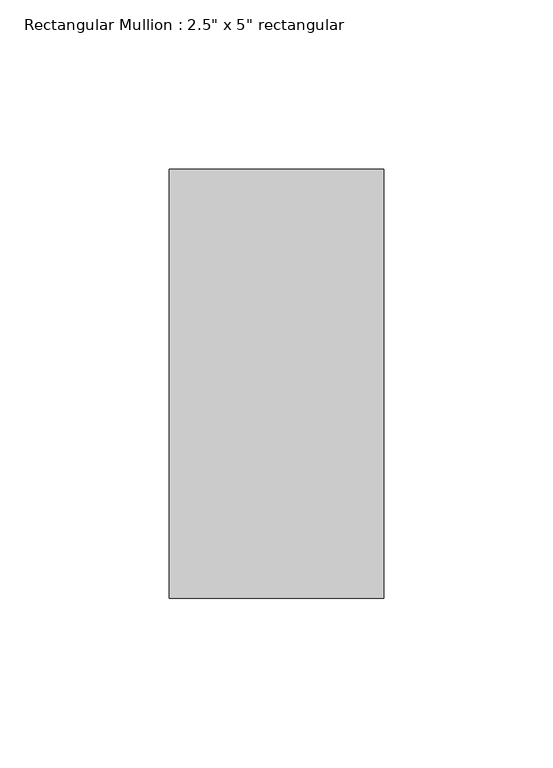
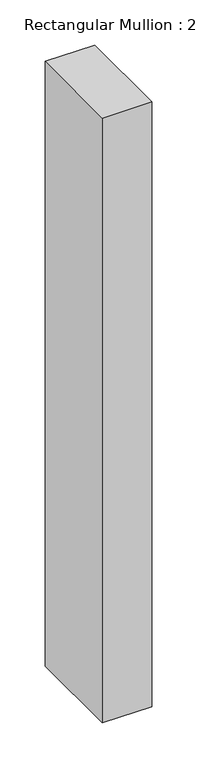
"""IFC4 building model written with IfcOpenShell, lengths in millimetres: member geometry."""

from ifc_helpers import new_model, si_unit, frame, origin, place, context, project, spatial, polyline, outline, extrude, source, transform, mapped, element, save


def member_a085fe98(model_context):
    return source(origin(), model_context, "Body", "SweptSolid", [
        extrude(outline(polyline([(31.75, 63.5), (31.75, -63.5), (-31.75, -63.5), (-31.75, 63.5), (31.75, 63.5)])), frame((0.0, 0.0, -819.1500001), z_axis=(0.0, 0.0, 1.0), x_axis=(1.0, 0.0, 0.0)), (0.0, 0.0, 1.0), 819.1500001),
    ])


if __name__ == "__main__":
    model = new_model("IFC4")
    model_context = context("Model", 3, world=origin())
    ifc_project = project(units=[si_unit("LENGTHUNIT", "METRE", prefix="MILLI")], contexts=[model_context])
    site = spatial("IfcSite", under=ifc_project)
    building = spatial("IfcBuilding", under=site)
    placement = place(None, origin())
    member_shape = member_a085fe98(model_context)
    element("IfcMember", 1, ObjectType="Rectangular Mullion : 2.5\" x 5\" rectangular", at=placement, inside=building, context=model_context, shape_type="MappedRepresentation", body=[
        mapped(member_shape, transform((0.0, 0.0, 0.0), x_axis=(1.0, 0.0, 0.0), y_axis=(0.0, 1.0, 0.0), z_axis=(0.0, 0.0, 1.0))),
    ])
    save(model, "model.ifc")

# Revit data of these elements
# Type "Rectangular Mullion : 2.5\" x 5\" rectangular"
#   built-in parameter 1007304 = 0.416667 (stored number, unit not read)
#   built-in parameter 1007301 = 0.104167 (stored number, unit not read)
#   built-in parameter 1007300 = 0.104167 (stored number, unit not read)
# Element 1 (IfcMember, "Rectangular Mullion : 2.5\" x 5\" rectangular")
#   Materials on its faces: "Aluminum"
# Materials
#   "Aluminum": class "Metal", colour RGB 247 247 247, transparency 0, Description = "Aluminum 6061", Cost = 0
